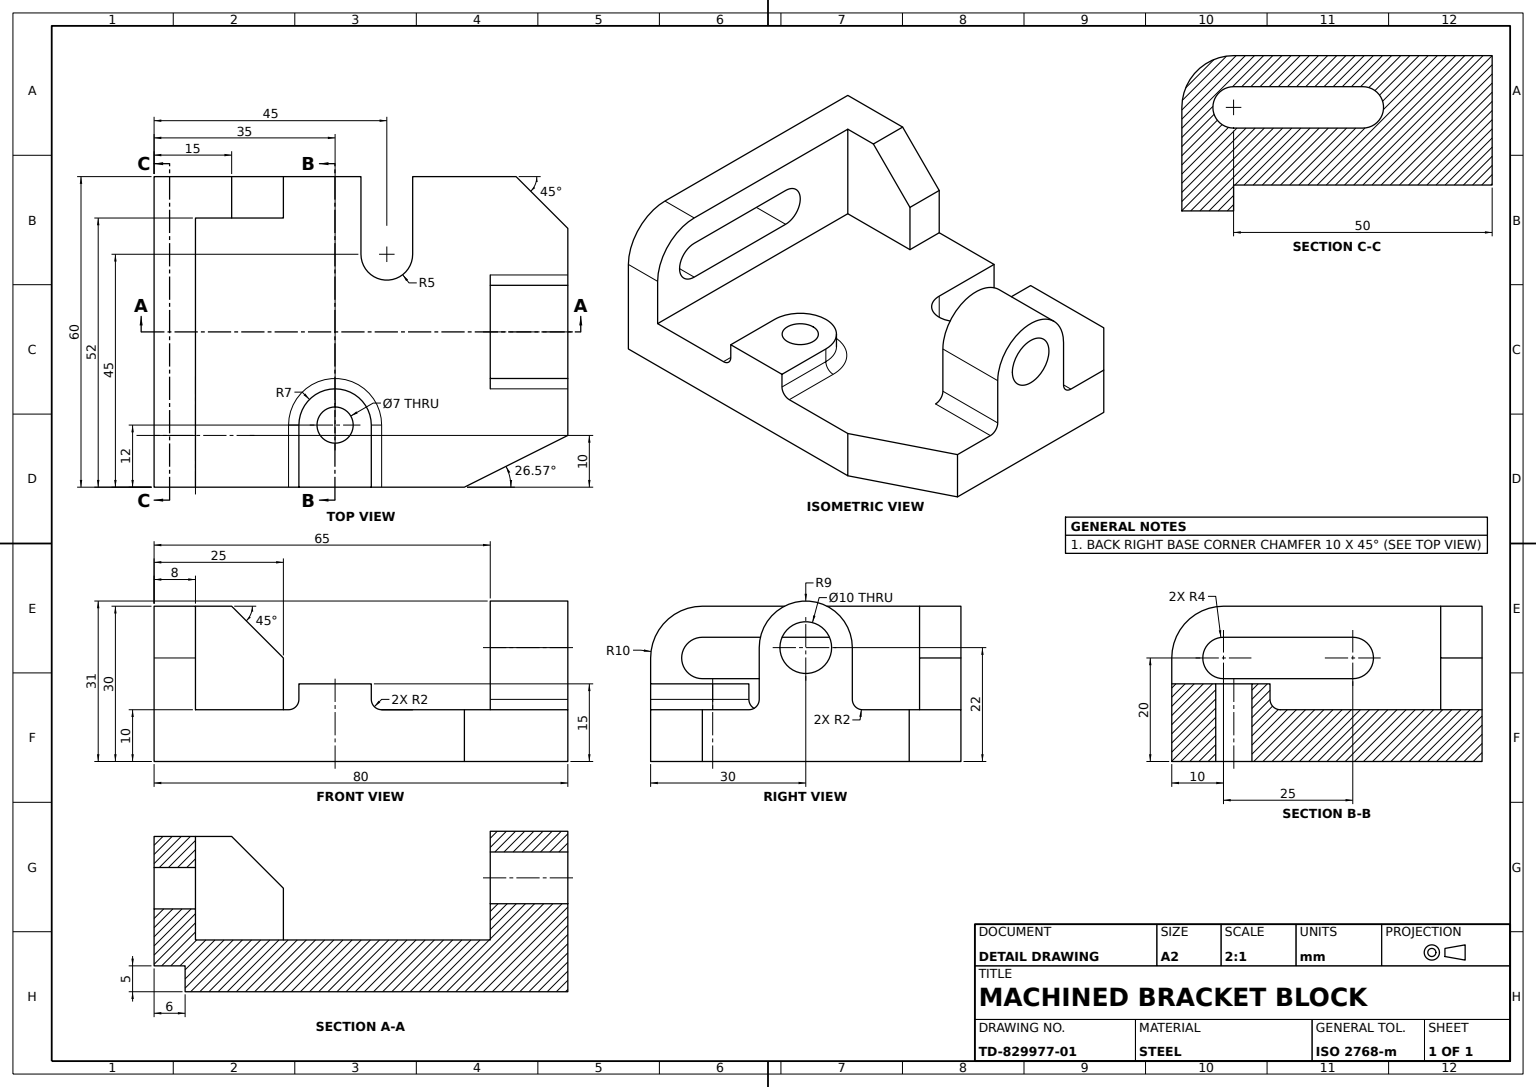
from build123d import *

# Parameters (mm, degrees)
BASE_PLATE_80X60X10_DEPTH      = 10
BASE_CORNER_CHAMFER_10_SIZE    = 10
SLOTTED_UPRIGHT_WALL_DEPTH     = 8
SIDE_BLOCK_SKETCH_W            = 17
SIDE_BLOCK_SKETCH_H            = 20
SIDE_BLOCK_25_DEPTH            = 8
SIDE_BLOCK_TOP_CHAMFER_10_SIZE = 10
HOLE_PAD_DEPTH                 = 5
PAD_HOLE_SKETCH_R              = 3.5
PAD_HOLE_7_DEPTH               = 87.746757864
PIVOT_LUG_SKETCH_R             = 5
PIVOT_LUG_DEPTH                = 15
LUG_ROOT_FILLET_R2_R           = 2
RELIEF_GROOVE_SKETCH_W         = 6
RELIEF_GROOVE_SKETCH_H         = 5
RELIEF_GROOVE_6X5_DEPTH        = 50


with BuildPart() as part:
    # Base Plate Sketch → Base Plate 80x60x10 (new body)
    with BuildSketch(Plane(origin=(0, 0, 0), x_dir=(1, 0, 0), z_dir=(0, 1, 0))):
        with BuildLine():
            Line((0, 0), (0, 30))
            Line((0, 30), (40, 30))
            Line((40, 30), (40, 15))
            ThreePointArc((40, 15), (45, 10), (50, 15))
            Line((50, 15), (50, 30))
            Line((50, 30), (80, 30))
            Line((80, 30), (80, -20))
            Line((80, -20), (60, -30))
            Line((60, -30), (0, -30))
            Line((0, -30), (0, 0))
        make_face()
    extrude(amount=BASE_PLATE_80X60X10_DEPTH)

    # Base Corner Chamfer 10
    base_corner_chamfer_10_edges = [part.edges().sort_by_distance(p)[0] for p in [
        (80, 5, -30),
    ]]
    chamfer(base_corner_chamfer_10_edges, length=BASE_CORNER_CHAMFER_10_SIZE)

    # Slotted Wall Sketch → Slotted Upright Wall (add)
    with BuildSketch(Plane.ZY):
        with BuildLine():
            Line((20, 30), (-30, 30))
            Line((-30, 30), (-30, 10))
            Line((-30, 10), (30, 10))
            Line((30, 10), (30, 20))
            ThreePointArc((30, 20), (27.071067812, 27.071067812), (20, 30))
        make_face()
        with BuildLine():
            Line((20, 16), (-5, 16))
            ThreePointArc((-5, 16), (-9, 20), (-5, 24))
            Line((-5, 24), (20, 24))
            ThreePointArc((20, 24), (24, 20), (20, 16))
        make_face(mode=Mode.SUBTRACT)
    extrude(amount=-SLOTTED_UPRIGHT_WALL_DEPTH)

    # Side Block Sketch → Side Block 25 (add)
    with BuildSketch(Plane(origin=(0, 0, -30), x_dir=(-1, 0, 0), z_dir=(0, 0, -1))):
        with Locations((-16.5, 20)):
            Rectangle(SIDE_BLOCK_SKETCH_W, SIDE_BLOCK_SKETCH_H)
    extrude(amount=-SIDE_BLOCK_25_DEPTH)

    # Side Block Top Chamfer 10
    side_block_top_chamfer_10_edges = [part.edges().sort_by_distance(p)[0] for p in [
        (25, 30, -26),
    ]]
    chamfer(side_block_top_chamfer_10_edges, length=SIDE_BLOCK_TOP_CHAMFER_10_SIZE)

    # Hole Pad Sketch → Hole Pad (add)
    with BuildSketch(Plane(origin=(0, 10, 0), x_dir=(1, 0, 0), z_dir=(0, 1, 0))):
        with BuildLine():
            Line((28, -18), (28, -30))
            Line((28, -30), (42, -30))
            Line((42, -30), (42, -18))
            ThreePointArc((42, -18), (35, -11), (28, -18))
        make_face()
    extrude(amount=HOLE_PAD_DEPTH)

    # Pad Hole Sketch → Pad Hole Ø7 (cut, through all)
    with BuildSketch(Plane(origin=(0, 15, 0), x_dir=(1, 0, 0), z_dir=(0, 1, 0))):
        with Locations(Location((35, -18, 0), (0, 0, 270))):
            Circle(PAD_HOLE_SKETCH_R)
    extrude(amount=-PAD_HOLE_7_DEPTH, mode=Mode.SUBTRACT)

    # Pivot Lug Sketch → Pivot Lug (add)
    with BuildSketch(Plane(origin=(80, 0, 0), x_dir=(0, 0, -1), z_dir=(1, 0, 0))):
        with BuildLine():
            Line((-9, 22), (-9, 10))
            Line((-9, 10), (9, 10))
            Line((9, 10), (9, 22))
            ThreePointArc((9, 22), (0, 31), (-9, 22))
        make_face()
        with Locations((0, 22)):
            Circle(PIVOT_LUG_SKETCH_R, mode=Mode.SUBTRACT)
    extrude(amount=-PIVOT_LUG_DEPTH)

    # Lug Root Fillet R2
    lug_root_fillet_r2_edges = [part.edges().sort_by_distance(p)[0] for p in [
        (72.5, 10, -9),
        (72.5, 10, 9),
        (35, 10, 11),
        (28, 10, 24),
        (42, 10, 24),
    ]]
    fillet(lug_root_fillet_r2_edges, radius=LUG_ROOT_FILLET_R2_R)

    # Relief Groove Sketch → Relief Groove 6x5 (cut)
    with BuildSketch(Plane(origin=(0, 0, -30), x_dir=(-1, 0, 0), z_dir=(0, 0, -1))):
        with Locations((-3, 2.5)):
            Rectangle(RELIEF_GROOVE_SKETCH_W, RELIEF_GROOVE_SKETCH_H)
    extrude(amount=-RELIEF_GROOVE_6X5_DEPTH, mode=Mode.SUBTRACT)


solid = part.part
